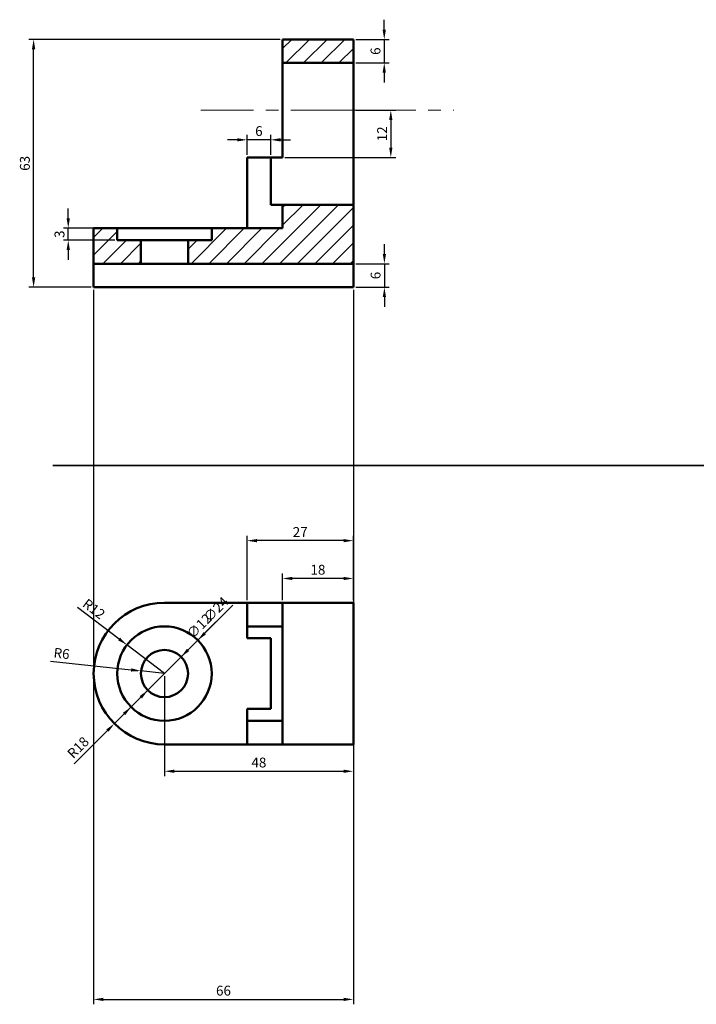
# Model space of a CAD drawing. Units: millimetres. Extents: x 2643 to 3341, y 1496 to 1804.
# Tile 1 of 2: x 2643 to 2815, y 1515 to 1765. Entities that reach past the tile are written whole.
import ezdxf

# ---------------------------------------------------------------- set-up
doc = ezdxf.new("R2010")
doc.units = ezdxf.units.MM
doc.linetypes.add('CENTER', pattern=[50.800000000000004, 31.75, -6.349999999999999, 6.349999999999999, -6.349999999999999])
for name, color, linetype, lineweight in [('M-CNTR', 1, 'CENTER', 18), ('M-DIMS', 2, 'Continuous', 25), ('M-HATC', 252, 'Continuous', 18), ('M-OUTL', 7, 'Continuous', 50), ('M-TTLB', 8, 'Continuous', 35)]:
    doc.layers.add(name, color=color, linetype=linetype, lineweight=lineweight)
doc.styles.get("Standard").update_dxf_attribs({"font": 'arial.ttf'})
doc.dimstyles.new('ISO-25', dxfattribs={"dimtxt": 2.5, "dimasz": 2.5, "dimexe": 1.25, "dimexo": 0.625, "dimtad": 1, "dimtxsty": 'Standard', "dimcen": 2.5, "dimadec": 0, "dimazin": 0, "dimtfac": 1, "dimtmove": 0, "dimatfit": 3, "dimfxl": 1, "dimarcsym": 0})

# ---------------------------------------------------------------- blocks, each defined once
blk = doc.blocks.new('*D1')
at = {"layer": 'Defpoints', "color": 0, "transparency": 16777216}
for p in [(2700.692987147304, 1734.597410231824), (2700.692987147304, 1730.12622113536), (2706.692987147304, 1730.12622113536)]:
    blk.add_point(p, dxfattribs=at)
at = {"layer": 'M-DIMS', "color": 0, "lineweight": -2, "transparency": 16777216}
for p, q in [((2698.192987147304, 1734.597410231824), (2695.692987147304, 1734.597410231824)), ((2700.692987147304, 1730.75122113536), (2700.692987147304, 1735.847410231824)), ((2706.692987147304, 1734.597410231824), (2700.692987147304, 1734.597410231824)), ((2706.692987147304, 1730.75122113536), (2706.692987147304, 1735.847410231824)), ((2709.192987147304, 1734.597410231824), (2711.692987147304, 1734.597410231824))]:
    blk.add_line(p, q, dxfattribs=at)
at = {"layer": 'M-DIMS', "color": 0, "transparency": 16777216}
for points in [[(2698.192987147304, 1735.01407689849), (2698.192987147304, 1734.180743565157), (2700.692987147304, 1734.597410231824)], [(2709.192987147304, 1735.01407689849), (2709.192987147304, 1734.180743565157), (2706.692987147304, 1734.597410231824)]]:
    blk.add_solid(points, dxfattribs=at)
at = {"layer": 'M-DIMS', "color": 0, "transparency": 16777216, "insert": (2703.692987147304, 1736.498842701128), "char_height": 2.5, "attachment_point": 5}
blk.add_mtext('6', dxfattribs=at)
blk = doc.blocks.new('*D2')
at = {"layer": 'Defpoints', "color": 0, "transparency": 16777216}
for p in [(2727.692987147305, 1703.126221135361), (2727.692987147305, 1697.126221135361), (2735.581009585733, 1697.126221135361)]:
    blk.add_point(p, dxfattribs=at)
at = {"layer": 'M-DIMS', "color": 0, "lineweight": -2, "transparency": 16777216}
for p, q in [((2735.581009585733, 1705.626221135361), (2735.581009585733, 1708.126221135361)), ((2728.317987147305, 1703.126221135361), (2736.831009585733, 1703.126221135361)), ((2735.581009585733, 1703.126221135361), (2735.581009585733, 1697.126221135361)), ((2728.317987147305, 1697.126221135361), (2736.831009585733, 1697.126221135361)), ((2735.581009585733, 1694.626221135361), (2735.581009585733, 1692.126221135361))]:
    blk.add_line(p, q, dxfattribs=at)
at = {"layer": 'M-DIMS', "color": 0, "transparency": 16777216}
for points in [[(2735.164342919067, 1705.626221135361), (2735.9976762524, 1705.626221135361), (2735.581009585733, 1703.126221135361)], [(2735.164342919067, 1694.626221135361), (2735.9976762524, 1694.626221135361), (2735.581009585733, 1697.126221135361)]]:
    blk.add_solid(points, dxfattribs=at)
at = {"layer": 'M-DIMS', "color": 0, "transparency": 16777216, "insert": (2733.679577116429, 1700.12622113536), "char_height": 2.5, "attachment_point": 5, "rotation": 90}
blk.add_mtext('6', dxfattribs=at)
blk = doc.blocks.new('*D3')
at = {"layer": 'Defpoints', "color": 0, "transparency": 16777216}
for p in [(2655.242849151799, 1712.126221135361), (2667.692987147305, 1712.126221135361), (2667.692987147305, 1709.126221135361)]:
    blk.add_point(p, dxfattribs=at)
at = {"layer": 'M-DIMS', "color": 0, "lineweight": -2, "transparency": 16777216}
for p, q in [((2655.242849151799, 1714.626221135361), (2655.242849151799, 1717.126221135361)), ((2667.067987147305, 1712.126221135361), (2653.992849151799, 1712.126221135361)), ((2655.242849151799, 1709.126221135361), (2655.242849151799, 1712.126221135361)), ((2667.067987147305, 1709.126221135361), (2653.992849151799, 1709.126221135361)), ((2655.242849151799, 1706.626221135361), (2655.242849151799, 1704.126221135361))]:
    blk.add_line(p, q, dxfattribs=at)
at = {"layer": 'M-DIMS', "color": 0, "transparency": 16777216}
for points in [[(2654.826182485132, 1714.626221135361), (2655.659515818465, 1714.626221135361), (2655.242849151799, 1712.126221135361)], [(2654.826182485132, 1706.626221135361), (2655.659515818465, 1706.626221135361), (2655.242849151799, 1709.126221135361)]]:
    blk.add_solid(points, dxfattribs=at)
at = {"layer": 'M-DIMS', "color": 0, "transparency": 16777216, "insert": (2653.340564022194, 1710.62622113536), "char_height": 2.5, "attachment_point": 5, "rotation": 90}
blk.add_mtext('3', dxfattribs=at)
blk = doc.blocks.new('*D4')
at = {"layer": 'Defpoints', "color": 0, "transparency": 16777216}
for p in [(2727.692987147305, 1760.126221135361), (2727.692987147305, 1754.126221135361), (2735.547727683754, 1754.126221135361)]:
    blk.add_point(p, dxfattribs=at)
at = {"layer": 'M-DIMS', "color": 0, "lineweight": -2, "transparency": 16777216}
for p, q in [((2735.547727683754, 1762.626221135361), (2735.547727683754, 1765.126221135361)), ((2728.317987147305, 1760.126221135361), (2736.797727683754, 1760.126221135361)), ((2735.547727683754, 1760.126221135361), (2735.547727683754, 1754.126221135361)), ((2728.317987147305, 1754.126221135361), (2736.797727683754, 1754.126221135361)), ((2735.547727683754, 1751.626221135361), (2735.547727683754, 1749.126221135361))]:
    blk.add_line(p, q, dxfattribs=at)
at = {"layer": 'M-DIMS', "color": 0, "transparency": 16777216}
for points in [[(2735.131061017087, 1762.626221135361), (2735.96439435042, 1762.626221135361), (2735.547727683754, 1760.126221135361)], [(2735.131061017087, 1751.626221135361), (2735.96439435042, 1751.626221135361), (2735.547727683754, 1754.126221135361)]]:
    blk.add_solid(points, dxfattribs=at)
at = {"layer": 'M-DIMS', "color": 0, "transparency": 16777216, "insert": (2733.64629521445, 1757.126221135359), "char_height": 2.5, "attachment_point": 5, "rotation": 90}
blk.add_mtext('6', dxfattribs=at)
blk = doc.blocks.new('*D5')
at = {"layer": 'Defpoints', "color": 0, "transparency": 16777216}
for p in [(2727.692987147305, 1742.126221135361), (2709.692987147305, 1730.126221135361), (2737.211378360657, 1730.126221135361)]:
    blk.add_point(p, dxfattribs=at)
at = {"layer": 'M-DIMS', "color": 0, "lineweight": -2, "transparency": 16777216}
for p, q in [((2728.317987147305, 1742.126221135361), (2738.461378360657, 1742.126221135361)), ((2737.211378360657, 1739.626221135361), (2737.211378360657, 1732.626221135361)), ((2710.317987147305, 1730.126221135361), (2738.461378360657, 1730.126221135361))]:
    blk.add_line(p, q, dxfattribs=at)
at = {"layer": 'M-DIMS', "color": 0, "transparency": 16777216}
for points in [[(2736.79471169399, 1739.626221135361), (2737.628045027323, 1739.626221135361), (2737.211378360657, 1742.126221135361)], [(2736.79471169399, 1732.626221135361), (2737.628045027323, 1732.626221135361), (2737.211378360657, 1730.126221135361)]]:
    blk.add_solid(points, dxfattribs=at)
at = {"layer": 'M-DIMS', "color": 0, "transparency": 16777216, "insert": (2735.331262398855, 1736.12622113536), "char_height": 2.5, "attachment_point": 5, "rotation": 90}
blk.add_mtext('12', dxfattribs=at)
blk = doc.blocks.new('*D6')
at = {"layer": 'Defpoints', "color": 0, "transparency": 16777216}
for p in [(2709.692987147304, 1623.146459531316), (2709.692987147304, 1616.984635921377), (2727.692987147304, 1616.984635921377)]:
    blk.add_point(p, dxfattribs=at)
at = {"layer": 'M-DIMS', "color": 0, "lineweight": -2, "transparency": 16777216}
for p, q in [((2709.692987147304, 1617.609635921376), (2709.692987147304, 1624.396459531316)), ((2727.692987147304, 1617.609635921376), (2727.692987147304, 1624.396459531316)), ((2725.192987147304, 1623.146459531316), (2712.192987147304, 1623.146459531316))]:
    blk.add_line(p, q, dxfattribs=at)
at = {"layer": 'M-DIMS', "color": 0, "transparency": 16777216}
for points in [[(2712.192987147304, 1623.563126197982), (2712.192987147304, 1622.729792864649), (2709.692987147304, 1623.146459531316)], [(2725.192987147304, 1623.563126197982), (2725.192987147304, 1622.729792864649), (2727.692987147304, 1623.146459531316)]]:
    blk.add_solid(points, dxfattribs=at)
at = {"layer": 'M-DIMS', "color": 0, "transparency": 16777216, "insert": (2718.692987147304, 1625.04789200062), "char_height": 2.5, "attachment_point": 5}
blk.add_mtext('18', dxfattribs=at)
blk = doc.blocks.new('*D7')
at = {"layer": 'Defpoints', "color": 0, "transparency": 16777216}
for p in [(2700.692987147304, 1632.754242811707), (2700.692987147304, 1616.984635921377), (2727.692987147304, 1616.984635921377)]:
    blk.add_point(p, dxfattribs=at)
at = {"layer": 'M-DIMS', "color": 0, "lineweight": -2, "transparency": 16777216}
for p, q in [((2700.692987147304, 1617.609635921376), (2700.692987147304, 1634.004242811707)), ((2727.692987147304, 1617.609635921376), (2727.692987147304, 1634.004242811707)), ((2725.192987147304, 1632.754242811707), (2703.192987147304, 1632.754242811707))]:
    blk.add_line(p, q, dxfattribs=at)
at = {"layer": 'M-DIMS', "color": 0, "transparency": 16777216}
for points in [[(2703.192987147304, 1633.170909478374), (2703.192987147304, 1632.33757614504), (2700.692987147304, 1632.754242811707)], [(2725.192987147304, 1633.170909478374), (2725.192987147304, 1632.33757614504), (2727.692987147304, 1632.754242811707)]]:
    blk.add_solid(points, dxfattribs=at)
at = {"layer": 'M-DIMS', "color": 0, "transparency": 16777216, "insert": (2714.192987147304, 1634.634358773508), "char_height": 2.5, "attachment_point": 5}
blk.add_mtext('27', dxfattribs=at)
blk = doc.blocks.new('*D14')
at = {"layer": 'Defpoints', "color": 0, "transparency": 16777216}
for p in [(2670.147204701232, 1606.256364566772), (2679.692987147304, 1598.984635921376)]:
    blk.add_point(p, dxfattribs=at)
at = {"layer": 'M-DIMS', "color": 0, "lineweight": -2, "transparency": 16777216}
for p, q in [((2657.568330422604, 1615.838623636206), (2668.158500024967, 1607.771308034562)), ((2679.692987147304, 1598.984635921376), (2670.147204701232, 1606.256364566772))]:
    blk.add_line(p, q, dxfattribs=at)
at = {"layer": 'M-DIMS', "color": 0, "transparency": 16777216}
blk.add_solid([(2668.410990602931, 1608.10275881394), (2667.906009447002, 1607.439857255185), (2670.147204701232, 1606.256364566772)], dxfattribs=at)
at = {"layer": 'M-DIMS', "color": 0, "transparency": 16777216, "insert": (2661.570640376558, 1615.153261232938), "char_height": 2.5, "attachment_point": 5, "rotation": 322.70079324285587}
blk.add_mtext('R12', dxfattribs=at)
blk = doc.blocks.new('*D15')
at = {"layer": 'Defpoints', "color": 0, "transparency": 16777216}
for p in [(2673.728824579553, 1599.639437315263), (2679.692987147305, 1598.984635921378)]:
    blk.add_point(p, dxfattribs=at)
at = {"layer": 'M-DIMS', "color": 0, "lineweight": -2, "transparency": 16777216}
for p, q in [((2650.700118174002, 1602.167743491095), (2671.24375684299, 1599.912271229381)), ((2679.692987147305, 1598.984635921378), (2673.728824579553, 1599.639437315263))]:
    blk.add_line(p, q, dxfattribs=at)
at = {"layer": 'M-DIMS', "color": 0, "transparency": 16777216}
blk.add_solid([(2671.28922916201, 1600.326449185475), (2671.198284523971, 1599.498093273287), (2673.728824579553, 1599.639437315263)], dxfattribs=at)
at = {"layer": 'M-DIMS', "color": 0, "transparency": 16777216, "insert": (2653.531697076077, 1603.769724137215), "char_height": 2.5, "attachment_point": 5, "rotation": 353.73462815325354}
blk.add_mtext('R6', dxfattribs=at)
blk = doc.blocks.new('*D16')
at = {"layer": 'Defpoints', "color": 0, "transparency": 16777216}
for p in [(2679.692987147305, 1598.984635921378), (2727.692987147304, 1598.984635921378), (2727.692987147304, 1574.162124802768)]:
    blk.add_point(p, dxfattribs=at)
at = {"layer": 'M-DIMS', "color": 0, "lineweight": -2, "transparency": 16777216}
for p, q in [((2679.692987147305, 1598.359635921378), (2679.692987147305, 1572.912124802768)), ((2727.692987147304, 1598.359635921378), (2727.692987147304, 1572.912124802768)), ((2682.192987147305, 1574.162124802768), (2725.192987147304, 1574.162124802768))]:
    blk.add_line(p, q, dxfattribs=at)
at = {"layer": 'M-DIMS', "color": 0, "transparency": 16777216}
for points in [[(2682.192987147305, 1574.578791469435), (2682.192987147305, 1573.745458136101), (2679.692987147305, 1574.162124802768)], [(2725.192987147304, 1574.578791469435), (2725.192987147304, 1573.745458136101), (2727.692987147304, 1574.162124802768)]]:
    blk.add_solid(points, dxfattribs=at)
at = {"layer": 'M-DIMS', "color": 0, "transparency": 16777216, "insert": (2703.692987147304, 1576.063557272072), "char_height": 2.5, "attachment_point": 5}
blk.add_mtext('48', dxfattribs=at)
blk = doc.blocks.new('*D33')
at = {"layer": 'Defpoints', "color": 0, "transparency": 16777216}
for p in [(2661.692987, 1697.126221), (2727.692987, 1697.126221), (2727.692987, 1516.199188)]:
    blk.add_point(p, dxfattribs=at)
at = {"layer": 'M-DIMS', "color": 0, "lineweight": -2, "transparency": 16777216}
for p, q in [((2661.692987, 1696.501221), (2661.692987, 1514.949188)), ((2727.692987, 1696.501221), (2727.692987, 1514.949188)), ((2664.192987, 1516.199188), (2725.192987, 1516.199188))]:
    blk.add_line(p, q, dxfattribs=at)
at = {"layer": 'M-DIMS', "color": 0, "transparency": 16777216}
for points in [[(2664.192987, 1516.615854666667), (2664.192987, 1515.782521333333), (2661.692987, 1516.199188)], [(2725.192987, 1516.615854666667), (2725.192987, 1515.782521333333), (2727.692987, 1516.199188)]]:
    blk.add_solid(points, dxfattribs=at)
at = {"layer": 'M-DIMS', "color": 0, "transparency": 16777216, "insert": (2694.692987, 1518.100620469304), "char_height": 2.5, "attachment_point": 5}
blk.add_mtext('66', dxfattribs=at)
blk = doc.blocks.new('*D34')
at = {"layer": 'Defpoints', "color": 0, "transparency": 16777216}
for p in [(2646.442987000002, 1760.126221000001), (2709.692987000001, 1760.126221000001), (2661.692987000001, 1697.126221000001)]:
    blk.add_point(p, dxfattribs=at)
at = {"layer": 'M-DIMS', "color": 0, "lineweight": -2, "transparency": 16777216}
for p, q in [((2709.067987000001, 1760.126221000001), (2645.192987000002, 1760.126221000001)), ((2646.442987000002, 1699.626221000001), (2646.442987000002, 1757.626221000001)), ((2661.067987000001, 1697.126221000001), (2645.192987000002, 1697.126221000001))]:
    blk.add_line(p, q, dxfattribs=at)
at = {"layer": 'M-DIMS', "color": 0, "transparency": 16777216}
for points in [[(2646.026320333335, 1757.626221000001), (2646.859653666668, 1757.626221000001), (2646.442987000002, 1760.126221000001)], [(2646.026320333335, 1699.626221000001), (2646.859653666668, 1699.626221000001), (2646.442987000002, 1697.126221000001)]]:
    blk.add_solid(points, dxfattribs=at)
at = {"layer": 'M-DIMS', "color": 0, "transparency": 16777216, "insert": (2644.540701870397, 1728.626221), "char_height": 2.5, "attachment_point": 5, "rotation": 90}
blk.add_mtext('63', dxfattribs=at)
blk = doc.blocks.new('*D37')
at = {"layer": 'Defpoints', "color": 0, "transparency": 16777216}
for p in [(2688.179093000001, 1607.469093), (2671.206880999999, 1590.500179)]:
    blk.add_point(p, dxfattribs=at)
at = {"layer": 'M-DIMS', "color": 0, "lineweight": -2, "transparency": 16777216}
for p, q in [((2697.047729639447, 1616.336006306998), (2689.947031715452, 1609.236688173791)), ((2671.206880999999, 1590.500179), (2688.179093000001, 1607.469093)), ((2669.438942284548, 1588.732583826209), (2667.671003569097, 1586.964988652418))]:
    blk.add_line(p, q, dxfattribs=at)
at = {"layer": 'M-DIMS', "color": 0, "transparency": 16777216}
for points in [[(2689.65243251982, 1609.531344626367), (2690.241630911084, 1608.942031721216), (2688.179093000001, 1607.469093)], [(2669.144343088916, 1589.027240278784), (2669.73354148018, 1588.437927373634), (2671.206880999999, 1590.500179)]]:
    blk.add_solid(points, dxfattribs=at)
at = {"layer": 'M-DIMS', "color": 0, "transparency": 16777216, "insert": (2692.987530102772, 1615.064235656117), "char_height": 2.5, "attachment_point": 5, "rotation": 44.99443266907718}
blk.add_mtext('∅24', dxfattribs=at)
blk = doc.blocks.new('*D38')
at = {"layer": 'Defpoints', "color": 0, "transparency": 16777216}
for p in [(2683.931449000001, 1603.231452), (2675.454524999999, 1594.73782)]:
    blk.add_point(p, dxfattribs=at)
at = {"layer": 'M-DIMS', "color": 0, "lineweight": -2, "transparency": 16777216}
for p, q in [((2692.779647238365, 1612.097090019134), (2685.697474679707, 1605.000958512737)), ((2675.454524999999, 1594.73782), (2683.931449000001, 1603.231452)), ((2673.688499320293, 1592.968313487263), (2671.922473640587, 1591.198806974526))]:
    blk.add_line(p, q, dxfattribs=at)
at = {"layer": 'M-DIMS', "color": 0, "transparency": 16777216}
for points in [[(2685.402556927584, 1605.295296126021), (2685.992392431829, 1604.706620899452), (2683.931449000001, 1603.231452)], [(2673.39358156817, 1593.262651100547), (2673.983417072415, 1592.673975873978), (2675.454524999999, 1594.73782)]]:
    blk.add_solid(points, dxfattribs=at)
at = {"layer": 'M-DIMS', "color": 0, "transparency": 16777216, "insert": (2688.726246698804, 1610.826359845455), "char_height": 2.5, "attachment_point": 5, "rotation": 45.05640932299194}
blk.add_mtext('∅12', dxfattribs=at)
blk = doc.blocks.new('*D39')
at = {"layer": 'Defpoints', "color": 0, "transparency": 16777216}
for p in [(2679.692987, 1598.984635999999), (2666.960889999999, 1586.260889999999)]:
    blk.add_point(p, dxfattribs=at)
at = {"layer": 'M-DIMS', "color": 0, "lineweight": -2, "transparency": 16777216}
for p, q in [((2679.692987, 1598.984635999999), (2666.960889999999, 1586.260889999999)), ((2656.765007714537, 1576.071695207805), (2665.192543211608, 1584.493703072708))]:
    blk.add_line(p, q, dxfattribs=at)
at = {"layer": 'M-DIMS', "color": 0, "transparency": 16777216}
blk.add_solid([(2664.89801205706, 1584.78842753744), (2665.487074366157, 1584.198978607976), (2666.960889999999, 1586.260889999999)], dxfattribs=at)
at = {"layer": 'M-DIMS', "color": 0, "transparency": 16777216, "insert": (2657.977557232999, 1579.971599274277), "char_height": 2.5, "attachment_point": 5, "rotation": 44.98120364595382}
blk.add_mtext('R18', dxfattribs=at)

msp = doc.modelspace()

# ---------------------------------------------------------------- hatches: boundary and pattern name
at = {"layer": 'M-HATC'}
h = msp.add_hatch(dxfattribs=at)
h.set_pattern_fill('ANSI31', color=256)
h.set_pattern_definition([(45, (0, 0), (-2.245064030267288, 2.245064030267288), [])])
h.paths.add_polyline_path([(2727.692987147304, 1754.12622113536), (2727.692987147304, 1760.12622113536), (2709.692987147304, 1760.12622113536), (2709.692987147304, 1754.12622113536)])
h.paths.add_polyline_path([(2727.692987147304, 1703.12622113536), (2727.692987147304, 1718.12622113536), (2709.692987147304, 1718.12622113536), (2709.692987147304, 1712.12622113536), (2691.692987147304, 1712.12622113536), (2691.692987147304, 1709.12622113536), (2685.692987147304, 1709.12622113536), (2685.692987147304, 1703.12622113536)])
h.paths.add_polyline_path([(2673.692987147303, 1703.12622113536), (2673.692987147304, 1709.12622113536), (2667.692987147304, 1709.12622113536), (2667.692987147304, 1712.12622113536), (2661.692987147304, 1712.12622113536), (2661.692987147304, 1703.12622113536)])

# ---------------------------------------------------------------- linework, layer by layer
at = {"layer": 'M-CNTR'}
msp.add_line((2727.692987147304, 1754.12622113536), (2727.692987147304, 1748.12622113536), dxfattribs=at)
at = {"layer": 'M-CNTR', "ltscale": 0.5}
for q in [(2688.897255867532, 1742.12622113536), (2753.266538247206, 1742.12622113536)]:
    msp.add_line((2727.692987147304, 1742.12622113536), q, dxfattribs=at)
at = {"layer": 'M-OUTL'}
for p, q in [((2727.692987147304, 1760.12622113536), (2709.692987147304, 1760.12622113536)), ((2709.692987147304, 1760.12622113536), (2709.692987147304, 1730.12622113536)), ((2727.692987147304, 1697.12622113536), (2727.692987147304, 1760.12622113536)), ((2727.692987147304, 1754.12622113536), (2709.692987147304, 1754.12622113536)), ((2709.692987147304, 1730.12622113536), (2700.692987147304, 1730.12622113536)), ((2700.692987147304, 1730.12622113536), (2700.692987147304, 1712.12622113536)), ((2706.692987147304, 1718.12622113536), (2706.692987147304, 1730.12622113536)), ((2709.692987147304, 1718.12622113536), (2706.692987147304, 1718.12622113536)), ((2709.692987147304, 1718.12622113536), (2709.692987147304, 1712.12622113536)), ((2709.692987147304, 1718.12622113536), (2727.692987147304, 1718.12622113536)), ((2661.692987147304, 1712.12622113536), (2679.692987147304, 1712.12622113536)), ((2661.692987147304, 1697.12622113536), (2661.692987147304, 1712.12622113536)), ((2667.692987147304, 1709.12622113536), (2667.692987147304, 1712.12622113536)), ((2679.692987147304, 1712.12622113536), (2709.692987147304, 1712.12622113536)), ((2691.692987147304, 1709.12622113536), (2691.692987147304, 1712.12622113536)), ((2667.692987147304, 1709.12622113536), (2679.692987147304, 1709.12622113536)), ((2673.692987147303, 1703.12622113536), (2673.692987147304, 1709.12622113536)), ((2679.692987147304, 1709.12622113536), (2691.692987147304, 1709.12622113536)), ((2685.692987147304, 1703.12622113536), (2685.692987147304, 1709.12622113536)), ((2661.692987147304, 1703.12622113536), (2679.692987147304, 1703.12622113536)), ((2679.692987147304, 1703.12622113536), (2727.692987147304, 1703.12622113536)), ((2661.692987147304, 1697.12622113536), (2679.692987147304, 1697.12622113536)), ((2679.692987147304, 1697.12622113536), (2727.692987147304, 1697.12622113536)), ((2679.692987147304, 1616.984635921377), (2727.692987147304, 1616.984635921377)), ((2700.692987147304, 1616.984635921377), (2700.692987147303, 1607.984635921377)), ((2709.692987147304, 1616.984635921377), (2709.692987147304, 1580.984635921377)), ((2709.692987147304, 1616.984635921377), (2709.692987147304, 1580.984635921377)), ((2727.692987147304, 1616.984635921377), (2727.692987147304, 1580.984635921377)), ((2709.692987147304, 1610.984635921376), (2700.692987147304, 1610.984635921376)), ((2706.692987147304, 1607.984635921377), (2700.692987147304, 1607.984635921377)), ((2706.692987147303, 1607.984635921376), (2706.692987147303, 1589.984635921376)), ((2706.692987147303, 1607.984635921376), (2706.692987147304, 1589.984635921376)), ((2706.692987147304, 1589.984635921376), (2700.692987147304, 1589.984635921376)), ((2700.692987147303, 1589.984635921376), (2700.692987147304, 1580.984635921377)), ((2709.692987147304, 1586.984635921377), (2700.692987147304, 1586.984635921377)), ((2679.692987147304, 1580.984635921377), (2727.692987147304, 1580.984635921377))]:
    msp.add_line(p, q, dxfattribs=at)
for radius in [12, 6]:
    msp.add_circle((2679.692987147304, 1598.984635921376), radius, dxfattribs=at)
msp.add_arc((2679.692987147304, 1598.984635921376), 18, 90, 270, dxfattribs=at)
at = {"layer": 'M-TTLB'}
msp.add_line((2818.579943598263, 1651.821496645129), (2651.296863881127, 1651.821496645129), dxfattribs=at)

# ---------------------------------------------------------------- dimensions: what is measured, and where the dimension line sits
at = {"layer": 'M-DIMS'}
for base, p1, p2, override, picture, middle in [((2735.547727683754, 1754.126221135361), (2727.692987147304, 1760.12622113536), (2727.692987147304, 1754.12622113536), {"dimclrd": 0, "dimclre": 0, "dimclrt": 0}, '*D4', (2733.64629521445, 1757.126221135359)), ((2646.442987000002, 1760.126221000001), (2661.692987, 1697.126221), (2709.692987, 1760.126221), {"dimdec": 0, "dimlfac": 1, "dimrnd": 0, "dimzin": 0, "dimdsep": 46, "dimlunit": 2}, '*D34', (2644.540701870397, 1728.626221)), ((2737.211378360657, 1730.126221135361), (2727.692987147304, 1742.12622113536), (2709.692987147304, 1730.12622113536), {"dimclrd": 0, "dimclre": 0, "dimclrt": 0}, '*D5', (2735.331262398855, 1736.12622113536)), ((2655.242849151799, 1712.126221135361), (2667.692987147304, 1709.12622113536), (2667.692987147304, 1712.12622113536), {"dimclrd": 0, "dimclre": 0, "dimclrt": 0}, '*D3', (2653.340564022194, 1710.62622113536)), ((2735.581009585733, 1697.126221135361), (2727.692987147304, 1703.12622113536), (2727.692987147304, 1697.12622113536), {"dimclrd": 0, "dimclre": 0, "dimclrt": 0}, '*D2', (2733.679577116429, 1700.12622113536))]:
    dim = msp.add_linear_dim(base=base, p1=p1, p2=p2, angle=90, dimstyle='ISO-25', override=override, dxfattribs=at)
    dim.commit()
    dim.dimension.update_dxf_attribs({"geometry": picture, "text_midpoint": middle})
for base, p1, p2, override, picture, middle in [((2700.692987147304, 1734.597410231824), (2706.692987147304, 1730.12622113536), (2700.692987147304, 1730.12622113536), {"dimclrd": 0, "dimclre": 0, "dimclrt": 0}, '*D1', (2703.692987147304, 1736.498842701128)), ((2727.692987, 1516.199188), (2661.692987, 1697.126221), (2727.692987, 1697.126221), {"dimdec": 0, "dimlfac": 1, "dimrnd": 0, "dimzin": 0, "dimdsep": 46, "dimlunit": 2}, '*D33', (2694.692987, 1518.100620469304)), ((2700.692987147304, 1632.754242811707), (2727.692987147304, 1616.984635921377), (2700.692987147304, 1616.984635921377), {"dimclrd": 0, "dimclre": 0, "dimclrt": 0}, '*D7', (2714.192987147304, 1634.634358773508)), ((2709.692987147304, 1623.146459531316), (2727.692987147304, 1616.984635921377), (2709.692987147304, 1616.984635921377), {"dimclrd": 0, "dimclre": 0, "dimclrt": 0}, '*D6', (2718.692987147304, 1625.04789200062)), ((2727.692987147304, 1574.162124802768), (2679.692987147305, 1598.984635921378), (2727.692987147304, 1598.984635921378), {"dimclrd": 0, "dimclre": 0, "dimclrt": 0}, '*D16', (2703.692987147304, 1576.063557272072))]:
    dim = msp.add_linear_dim(base=base, p1=p1, p2=p2, dimstyle='ISO-25', override=override, dxfattribs=at)
    dim.commit()
    dim.dimension.update_dxf_attribs({"geometry": picture, "text_midpoint": middle})
for p1, p2, picture, middle in [((2671.206880999999, 1590.500179), (2688.179093000001, 1607.469093), '*D37', (2694.381350035175, 1613.67014482729)), ((2675.454524999999, 1594.73782), (2683.931449000001, 1603.231452), '*D38', (2690.121573798889, 1609.433777522304))]:
    dim = msp.add_diameter_dim_2p(p1=p1, p2=p2, dimstyle='ISO-25', override={"dimdec": 0, "dimlfac": 1, "dimrnd": 0, "dimzin": 0, "dimdsep": 46, "dimlunit": 2}, dxfattribs=at)
    dim.commit()
    dim.dimension.update_dxf_attribs({"geometry": picture, "text_midpoint": middle})
for center, mpoint, override, picture, middle in [((2679.692987147304, 1598.984635921376), (2670.147204701232, 1606.256364566772), {"dimclrd": 0, "dimclre": 0, "dimclrt": 0}, '*D14', (2660.43133261855, 1613.657663070877)), ((2679.692987147305, 1598.984635921378), (2673.728824579553, 1599.639437315263), {"dimclrd": 0, "dimclre": 0, "dimclrt": 0}, '*D15', (2653.324186970864, 1601.879648744127)), ((2679.692987, 1598.984635999999), (2666.960889999999, 1586.260889999999), {"dimdec": 0, "dimlfac": 1, "dimrnd": 0, "dimzin": 0, "dimdsep": 46, "dimlunit": 2}, '*D39', (2659.321631874151, 1578.626642474103))]:
    dim = msp.add_radius_dim(center=center, mpoint=mpoint, dimstyle='ISO-25', override=override, dxfattribs=at)
    dim.commit()
    dim.dimension.update_dxf_attribs({"geometry": picture, "text_midpoint": middle, "dimtype": 164})

doc.saveas('drawing.dxf')
